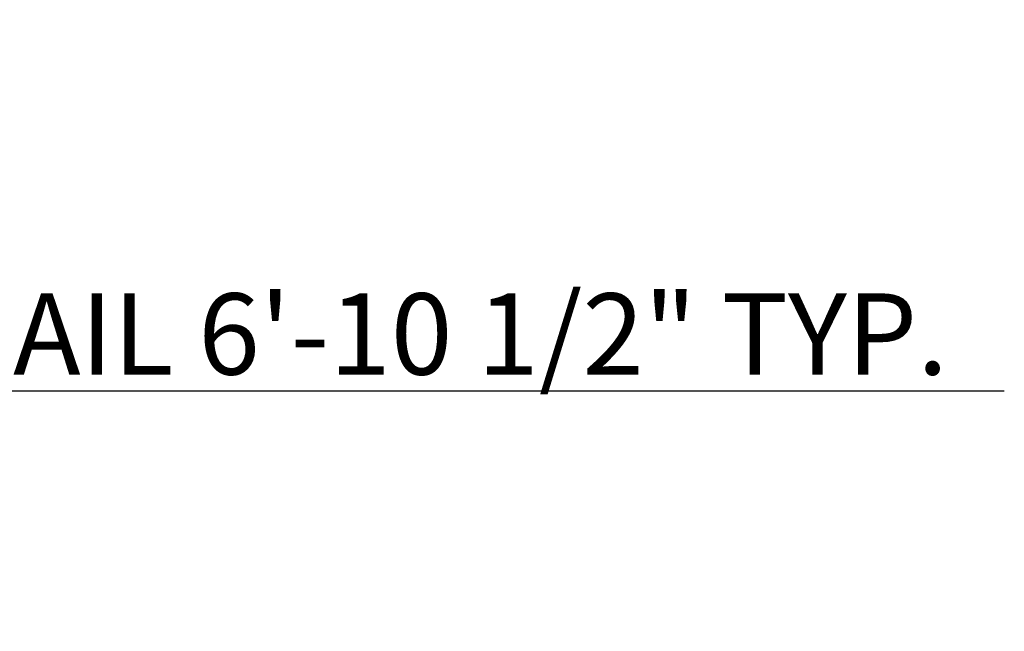
# Model space of a CAD drawing. Units: millimetres. Extents: x 542930 to 543750, y 628093 to 628738.
# Tile 14 of 14: x 543604 to 543750, y 628458 to 628548. Entities that reach past the tile are written whole.
import ezdxf

# ---------------------------------------------------------------- set-up
doc = ezdxf.new("R2010")
doc.units = ezdxf.units.MM
doc.layers.add('A-ANNO-DIMS', color=2, linetype='Continuous', lineweight=18)
doc.styles.get("Standard").update_dxf_attribs({"font": 'arial.ttf'})
doc.dimstyles.new('ISO-25', dxfattribs={"dimtxt": 12, "dimasz": 2.5, "dimexe": 1.25, "dimexo": 0.625, "dimtad": 1, "dimdec": 0, "dimlunit": 3, "dimtxsty": 'Standard', "dimcen": 2.5, "dimadec": 0, "dimazin": 0, "dimtfac": 1, "dimtdec": 0, "dimtmove": 0, "dimatfit": 3, "dimfxl": 1, "dimarcsym": 0})

# ---------------------------------------------------------------- blocks, each defined once
blk = doc.blocks.new('*D45')
at = {"layer": 'A-ANNO-DIMS', "color": 0, "lineweight": -2, "transparency": 16777216}
for p, q in [((543407.17, 628481.45), (543407.17, 628494.45)), ((543489.67, 628481.45), (543489.67, 628494.45)), ((543409.67, 628493.2), (543487.17, 628493.2)), ((543489.67, 628493.2), (543749.65, 628493.2))]:
    blk.add_line(p, q, dxfattribs=at)
at = {"layer": 'A-ANNO-DIMS', "color": 0, "transparency": 16777216}
for points in [[(543409.67, 628493.62), (543409.67, 628492.78), (543407.17, 628493.2)], [(543487.17, 628493.62), (543487.17, 628492.78), (543489.67, 628493.2)]]:
    blk.add_solid(points, dxfattribs=at)
at = {"layer": 'Defpoints', "color": 0, "transparency": 16777216}
for p in [(543489.67, 628493.2), (543407.17, 628480.83), (543489.67, 628480.83)]:
    blk.add_point(p, dxfattribs=at)
at = {"layer": 'A-ANNO-DIMS', "color": 0, "transparency": 16777216, "insert": (543620.91, 628500.03), "char_height": 12, "attachment_point": 5}
blk.add_mtext('WARDROBE RAIL 6\'-10 1/2" TYP.', dxfattribs=at)

msp = doc.modelspace()

# ---------------------------------------------------------------- dimensions: what is measured, and where the dimension line sits
at = {"layer": 'A-ANNO-DIMS'}
dim = msp.add_linear_dim(base=(543489.67, 628493.2), p1=(543407.17, 628480.83), p2=(543489.67, 628480.83), text='WARDROBE RAIL <> TYP.', dimstyle='ISO-25', override={"dimdec": 1, "dimlfac": 1, "dimrnd": 0, "dimzin": 1, "dimdsep": 46, "dimlunit": 4, "dimfrac": 2}, dxfattribs=at)
dim.commit()
dim.dimension.update_dxf_attribs({"geometry": '*D45', "text_midpoint": (543620.91, 628500.03)})

doc.saveas('drawing.dxf')
